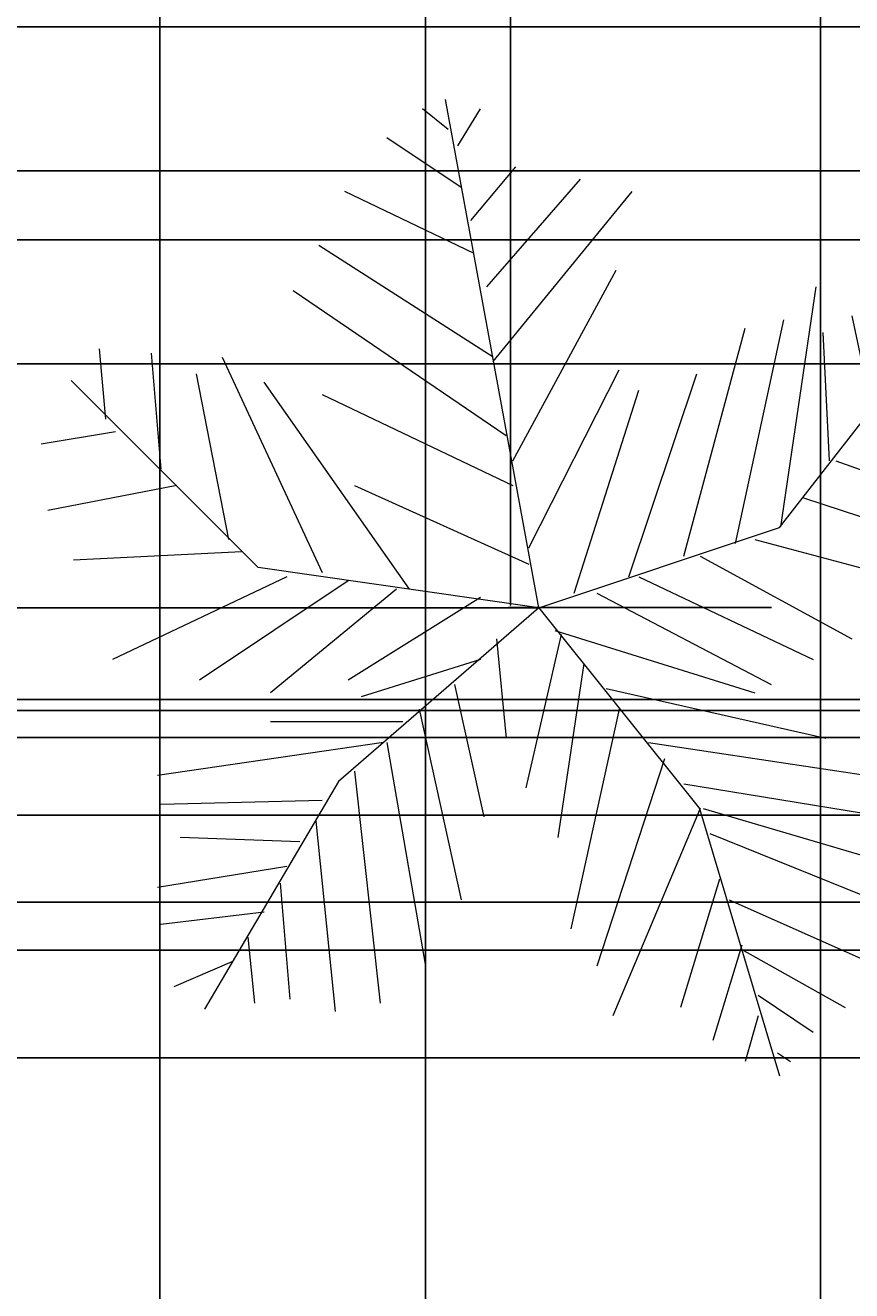
# Model space of a CAD drawing. Units: inches. Extents: x 818 to 1898, y 976 to 2364.
# Tile 10 of 96: x 1002 to 1071, y 1668 to 1773. Entities that reach past the tile are written whole.
import ezdxf

# ---------------------------------------------------------------- set-up
doc = ezdxf.new("R2010")
doc.units = ezdxf.units.IN
doc.header["$LTSCALE"] = 5
doc.header["$MEASUREMENT"] = 0
doc.layers.add('A-ANNO-DIMS', color=2, linetype='Continuous', lineweight=18)
doc.layers.add('L-PLNT', color=116, linetype='Continuous', lineweight=13, true_color=0x136734)
doc.styles.get("Standard").update_dxf_attribs({"font": 'arial.ttf'})
doc.dimstyles.get("Standard").update_dxf_attribs({"dimtxt": 0.18, "dimasz": 0.18, "dimexe": 0.18, "dimexo": 0.0625, "dimgap": 0.09, "dimtad": 0, "dimtih": 1, "dimtoh": 1, "dimdec": 4, "dimzin": 0, "dimdsep": 46, "dimtxsty": 'Standard', "dimcen": 0.09, "dimadec": 0, "dimazin": 0, "dimtfac": 1, "dimtdec": 4, "dimtofl": 0, "dimtmove": 0, "dimatfit": 3, "dimfxl": 1, "dimtolj": 1, "dimtzin": 0, "dimarcsym": 0})

# ---------------------------------------------------------------- blocks, each defined once
blk = doc.blocks.new('PALM-BORDER')
for p, q in [((41.53, 39.05), (33.72, 81.45)), ((33.95, 78.95), (31.8, 80.68)), ((34.76, 77.57), (36.65, 80.68)), ((35.03, 74.11), (28.83, 78.26)), ((35.84, 71.35), (39.61, 75.84)), ((37.18, 65.82), (45, 74.8)), ((36.11, 68.59), (25.33, 73.77)), ((37.72, 59.6), (49.31, 73.77)), ((37.72, 59.95), (23.17, 69.28)), ((39.34, 51.31), (47.96, 67.2)), ((38.8, 53.39), (21.02, 65.48)), ((61.61, 45.75), (77.23, 65.83)), ((61.71, 45.79), (64.67, 65.82)), ((74.37, 66.17), (75.18, 63.4)), ((70.33, 64.44), (72.75, 60.3)), ((67.63, 63.4), (69.25, 55.81)), ((53.62, 43.37), (58.74, 62.37)), ((57.93, 44.41), (61.97, 63.06)), ((65.21, 62.02), (65.75, 51.31)), ((74.1, 61.33), (79.49, 62.02)), ((5.39, 54.77), (4.85, 60.64)), ((9.16, 60.3), (9.97, 50.62)), ((15.09, 59.95), (23.44, 41.99)), ((12.93, 58.57), (15.63, 44.75)), ((40.69, 44.06), (48.23, 58.91)), ((49.04, 41.64), (54.7, 58.57)), ((71.68, 58.22), (77.87, 57.53)), ((18.1, 42.4), (2.48, 58.02)), ((30.72, 40.61), (18.59, 57.88)), ((44.46, 40.26), (49.85, 57.19)), ((23.44, 56.84), (39.34, 49.24)), ((6.2, 53.73), (0, 52.7)), ((68.44, 53.73), (77.33, 52.35)), ((66.29, 51.31), (77.87, 47.17)), ((11.32, 49.24), (0.54, 47.17)), ((26.14, 49.24), (40.69, 42.68)), ((63.59, 48.21), (77.33, 43.71)), ((41.53, 39.05), (61.61, 45.75)), ((59.55, 44.75), (76.26, 40.26)), ((16.71, 43.71), (2.69, 43.02)), ((54.97, 43.37), (67.63, 36.46)), ((41.53, 39.05), (18.1, 42.4)), ((20.48, 41.64), (5.93, 34.73)), ((25.6, 41.3), (13.2, 33.01)), ((49.85, 41.64), (64.4, 34.73)), ((29.64, 40.61), (19.13, 31.97)), ((46.35, 40.26), (60.9, 32.66)), ((36.65, 39.91), (25.6, 33.01)), ((41.53, 39.05), (24.79, 24.55)), ((41.53, 39.05), (54.92, 22.32)), ((42.84, 37.15), (59.55, 31.97)), ((37.99, 36.46), (38.8, 28.17)), ((43.38, 36.81), (40.42, 24.02)), ((36.65, 34.73), (26.68, 31.62)), ((45.27, 34.39), (43.11, 19.88)), ((34.49, 32.66), (36.92, 21.61)), ((47.15, 32.32), (65.48, 28.17)), ((31.53, 30.59), (35.03, 14.7)), ((48.23, 30.59), (44.19, 12.28)), ((30.18, 29.55), (19.13, 29.55)), ((28.56, 27.82), (9.7, 25.06)), ((28.83, 27.82), (32.07, 9.17)), ((50.66, 27.82), (68.98, 25.06)), ((52, 26.44), (46.35, 9.17)), ((26.14, 25.41), (28.29, 6.06)), ((24.79, 24.55), (13.63, 5.58)), ((53.62, 24.37), (68.44, 21.95)), ((23.44, 22.99), (9.97, 22.64)), ((54.97, 22.3), (47.69, 5.02)), ((54.92, 22.32), (61.61, 0)), ((55.24, 22.3), (71.68, 17.46)), ((22.9, 21.26), (24.52, 5.37)), ((55.78, 20.22), (70.33, 14.35)), ((21.56, 19.53), (11.59, 19.88)), ((20.48, 17.46), (9.7, 15.73)), ((19.94, 16.08), (20.75, 6.41)), ((56.59, 16.42), (53.35, 5.72)), ((57.39, 14.7), (70.6, 8.83)), ((18.59, 13.66), (9.97, 12.62)), ((17.24, 11.59), (17.78, 6.06)), ((58.47, 10.9), (56.05, 2.95)), ((15.9, 9.52), (11.05, 7.44)), ((58.47, 10.55), (67.09, 5.72)), ((59.82, 6.75), (64.4, 3.64)), ((59.82, 5.02), (58.74, 1.22)), ((61.44, 1.92), (62.51, 1.22))]:
    blk.add_line(p, q)
blk = doc.blocks.new('*D28')
at = {"layer": 'A-ANNO-DIMS', "color": 0, "lineweight": -2, "ltscale": 5, "transparency": 16777216}
for p, q in [((1064.25, 1870.18), (1042.3, 1870.18)), ((1042.48, 1870), (1042.48, 1797.61)), ((1042.48, 1724.84), (1042.48, 1797.24)), ((1064.25, 1724.66), (1042.3, 1724.66))]:
    blk.add_line(p, q, dxfattribs=at)
at = {"layer": 'A-ANNO-DIMS', "color": 0, "ltscale": 5, "transparency": 16777216}
for points in [[(1042.45, 1870), (1042.51, 1870), (1042.48, 1870.18)], [(1042.45, 1724.84), (1042.51, 1724.84), (1042.48, 1724.66)]]:
    blk.add_solid(points, dxfattribs=at)
at = {"layer": 'Defpoints', "color": 0, "ltscale": 5, "transparency": 16777216}
for p in [(1042.48, 1870.18), (1064.31, 1870.18), (1064.31, 1724.66)]:
    blk.add_point(p, dxfattribs=at)
at = {"layer": 'A-ANNO-DIMS', "color": 0, "ltscale": 5, "transparency": 16777216, "insert": (1042.48, 1797.42), "char_height": 0.18, "attachment_point": 5}
blk.add_mtext('\\A1;DECK PALM 146 TYP.', dxfattribs=at)
blk = doc.blocks.new('*D59')
at = {"layer": 'A-ANNO-DIMS', "color": 0, "lineweight": -2, "ltscale": 5, "transparency": 16777216}
for p, q in [((1251.64, 2300.39), (818.03, 2300.39)), ((818.21, 2300.21), (818.21, 1669.95)), ((818.21, 1039.32), (818.21, 1669.59)), ((896.05, 1039.14), (818.03, 1039.14))]:
    blk.add_line(p, q, dxfattribs=at)
at = {"layer": 'A-ANNO-DIMS', "color": 0, "ltscale": 5, "transparency": 16777216}
for points in [[(818.18, 2300.21), (818.24, 2300.21), (818.21, 2300.39)], [(818.18, 1039.32), (818.24, 1039.32), (818.21, 1039.14)]]:
    blk.add_solid(points, dxfattribs=at)
at = {"layer": 'Defpoints', "color": 0, "ltscale": 5, "transparency": 16777216}
for p in [(818.21, 2300.39), (1251.71, 2300.39), (896.11, 1039.14)]:
    blk.add_point(p, dxfattribs=at)
at = {"layer": 'A-ANNO-DIMS', "color": 0, "ltscale": 5, "transparency": 16777216, "insert": (818.21, 1669.77), "char_height": 0.18, "attachment_point": 5}
blk.add_mtext('\\A1;1261.2', dxfattribs=at)
blk = doc.blocks.new('*D79')
at = {"layer": 'A-ANNO-DIMS', "color": 0, "lineweight": -2, "ltscale": 5, "transparency": 16777216}
for p, q in [((992.73, 1203.03), (992.73, 2363.87)), ((992.91, 2363.69), (1032.01, 2363.69)), ((1071.55, 2363.69), (1032.44, 2363.69)), ((1071.73, 1203.03), (1071.73, 2363.87))]:
    blk.add_line(p, q, dxfattribs=at)
at = {"layer": 'A-ANNO-DIMS', "color": 0, "ltscale": 5, "transparency": 16777216}
for points in [[(992.91, 2363.72), (992.91, 2363.66), (992.73, 2363.69)], [(1071.55, 2363.72), (1071.55, 2363.66), (1071.73, 2363.69)]]:
    blk.add_solid(points, dxfattribs=at)
at = {"layer": 'Defpoints', "color": 0, "ltscale": 5, "transparency": 16777216}
for p in [(1071.73, 2363.69), (992.73, 1202.96), (1071.73, 1202.96)]:
    blk.add_point(p, dxfattribs=at)
at = {"layer": 'A-ANNO-DIMS', "color": 0, "ltscale": 5, "transparency": 16777216, "insert": (1032.23, 2363.69), "char_height": 0.18, "attachment_point": 5}
blk.add_mtext('\\A1;79', dxfattribs=at)
blk = doc.blocks.new('*D84')
at = {"layer": 'A-ANNO-DIMS', "color": 0, "lineweight": -2, "ltscale": 5, "transparency": 16777216}
for p, q in [((1197.66, 1700.08), (818.03, 1700.08)), ((818.21, 1699.9), (818.21, 1600.76)), ((818.21, 1501.26), (818.21, 1600.4)), ((1197.66, 1501.08), (818.03, 1501.08))]:
    blk.add_line(p, q, dxfattribs=at)
at = {"layer": 'A-ANNO-DIMS', "color": 0, "ltscale": 5, "transparency": 16777216}
for points in [[(818.18, 1699.9), (818.24, 1699.9), (818.21, 1700.08)], [(818.18, 1501.26), (818.24, 1501.26), (818.21, 1501.08)]]:
    blk.add_solid(points, dxfattribs=at)
at = {"layer": 'Defpoints', "color": 0, "ltscale": 5, "transparency": 16777216}
for p in [(818.21, 1700.08), (1197.73, 1700.08), (1197.73, 1501.08)]:
    blk.add_point(p, dxfattribs=at)
at = {"layer": 'A-ANNO-DIMS', "color": 0, "ltscale": 5, "transparency": 16777216, "insert": (818.21, 1600.58), "char_height": 0.18, "attachment_point": 5}
blk.add_mtext('\\A1;199', dxfattribs=at)
blk = doc.blocks.new('*D91')
at = {"layer": 'A-ANNO-DIMS', "color": 0, "lineweight": -2, "ltscale": 5, "transparency": 16777216}
for p, q in [((959.17, 1071.12), (959.17, 2363.87)), ((959.35, 2363.69), (985.8, 2363.69)), ((1013.04, 2363.69), (986.59, 2363.69)), ((1013.22, 1071.12), (1013.22, 2363.87))]:
    blk.add_line(p, q, dxfattribs=at)
at = {"layer": 'A-ANNO-DIMS', "color": 0, "ltscale": 5, "transparency": 16777216}
for points in [[(959.35, 2363.72), (959.35, 2363.66), (959.17, 2363.69)], [(1013.04, 2363.72), (1013.04, 2363.66), (1013.22, 2363.69)]]:
    blk.add_solid(points, dxfattribs=at)
at = {"layer": 'Defpoints', "color": 0, "ltscale": 5, "transparency": 16777216}
for p in [(1013.22, 2363.69), (959.17, 1071.06), (1013.22, 1071.06)]:
    blk.add_point(p, dxfattribs=at)
at = {"layer": 'A-ANNO-DIMS', "color": 0, "ltscale": 5, "transparency": 16777216, "insert": (986.2, 2363.69), "char_height": 0.18, "attachment_point": 5}
blk.add_mtext('\\A1;54.04', dxfattribs=at)
blk = doc.blocks.new('*D92')
at = {"layer": 'A-ANNO-DIMS', "color": 0, "lineweight": -2, "ltscale": 5, "transparency": 16777216}
for p, q in [((1013.22, 1071.12), (1013.22, 2363.87)), ((1013.4, 2363.69), (1040.38, 2363.69)), ((1068.16, 2363.69), (1041.17, 2363.69)), ((1068.34, 1071.12), (1068.34, 2363.87))]:
    blk.add_line(p, q, dxfattribs=at)
at = {"layer": 'A-ANNO-DIMS', "color": 0, "ltscale": 5, "transparency": 16777216}
for points in [[(1013.4, 2363.72), (1013.4, 2363.66), (1013.22, 2363.69)], [(1068.16, 2363.72), (1068.16, 2363.66), (1068.34, 2363.69)]]:
    blk.add_solid(points, dxfattribs=at)
at = {"layer": 'Defpoints', "color": 0, "ltscale": 5, "transparency": 16777216}
for p in [(1068.34, 2363.69), (1013.22, 1071.06), (1068.34, 1071.06)]:
    blk.add_point(p, dxfattribs=at)
at = {"layer": 'A-ANNO-DIMS', "color": 0, "ltscale": 5, "transparency": 16777216, "insert": (1040.78, 2363.69), "char_height": 0.18, "attachment_point": 5}
blk.add_mtext('\\A1;55.12', dxfattribs=at)
blk = doc.blocks.new('*D93')
at = {"layer": 'A-ANNO-DIMS', "color": 0, "lineweight": -2, "ltscale": 5, "transparency": 16777216}
for p, q in [((1068.34, 1071.12), (1068.34, 2363.87)), ((1068.52, 2363.69), (1094.16, 2363.69)), ((1120.58, 2363.69), (1094.94, 2363.69)), ((1120.76, 1071.12), (1120.76, 2363.87))]:
    blk.add_line(p, q, dxfattribs=at)
at = {"layer": 'A-ANNO-DIMS', "color": 0, "ltscale": 5, "transparency": 16777216}
for points in [[(1068.52, 2363.72), (1068.52, 2363.66), (1068.34, 2363.69)], [(1120.58, 2363.72), (1120.58, 2363.66), (1120.76, 2363.69)]]:
    blk.add_solid(points, dxfattribs=at)
at = {"layer": 'Defpoints', "color": 0, "ltscale": 5, "transparency": 16777216}
for p in [(1120.76, 2363.69), (1068.34, 1071.06), (1120.76, 1071.06)]:
    blk.add_point(p, dxfattribs=at)
at = {"layer": 'A-ANNO-DIMS', "color": 0, "ltscale": 5, "transparency": 16777216, "insert": (1094.55, 2363.69), "char_height": 0.18, "attachment_point": 5}
blk.add_mtext('\\A1;52.42', dxfattribs=at)
blk = doc.blocks.new('*D119')
at = {"layer": 'A-ANNO-DIMS', "color": 0, "lineweight": -2, "ltscale": 5, "transparency": 16777216}
for p, q in [((1766.29, 1716.99), (818.03, 1716.99)), ((818.21, 1716.81), (818.21, 1672.43)), ((818.21, 1627.69), (818.21, 1672.06)), ((1766.29, 1627.51), (818.03, 1627.51))]:
    blk.add_line(p, q, dxfattribs=at)
at = {"layer": 'A-ANNO-DIMS', "color": 0, "ltscale": 5, "transparency": 16777216}
for points in [[(818.18, 1716.81), (818.24, 1716.81), (818.21, 1716.99)], [(818.18, 1627.69), (818.24, 1627.69), (818.21, 1627.51)]]:
    blk.add_solid(points, dxfattribs=at)
at = {"layer": 'Defpoints', "color": 0, "ltscale": 5, "transparency": 16777216}
for p in [(818.21, 1716.99), (1766.35, 1716.99), (1766.35, 1627.51)]:
    blk.add_point(p, dxfattribs=at)
at = {"layer": 'A-ANNO-DIMS', "color": 0, "ltscale": 5, "transparency": 16777216, "insert": (818.21, 1672.25), "char_height": 0.18, "attachment_point": 5}
blk.add_mtext('\\A1;89.48', dxfattribs=at)
blk = doc.blocks.new('*D120')
at = {"layer": 'A-ANNO-DIMS', "color": 0, "lineweight": -2, "ltscale": 5, "transparency": 16777216}
for p, q in [((1766.29, 1797.72), (818.03, 1797.72)), ((818.21, 1797.54), (818.21, 1757.53)), ((818.21, 1717.17), (818.21, 1757.17)), ((1766.29, 1716.99), (818.03, 1716.99))]:
    blk.add_line(p, q, dxfattribs=at)
at = {"layer": 'A-ANNO-DIMS', "color": 0, "ltscale": 5, "transparency": 16777216}
for points in [[(818.18, 1797.54), (818.24, 1797.54), (818.21, 1797.72)], [(818.18, 1717.17), (818.24, 1717.17), (818.21, 1716.99)]]:
    blk.add_solid(points, dxfattribs=at)
at = {"layer": 'Defpoints', "color": 0, "ltscale": 5, "transparency": 16777216}
for p in [(818.21, 1797.72), (1766.35, 1797.72), (1766.35, 1716.99)]:
    blk.add_point(p, dxfattribs=at)
at = {"layer": 'A-ANNO-DIMS', "color": 0, "ltscale": 5, "transparency": 16777216, "insert": (818.21, 1757.35), "char_height": 0.18, "attachment_point": 5}
blk.add_mtext('\\A1;80.73', dxfattribs=at)
blk = doc.blocks.new('*D126')
at = {"layer": 'A-ANNO-DIMS', "color": 0, "lineweight": -2, "ltscale": 5, "transparency": 16777216}
for p, q in [((1035.38, 1252.09), (1035.38, 2363.87)), ((1035.56, 2363.69), (1075.41, 2363.69)), ((1116.01, 2363.69), (1076.16, 2363.69)), ((1116.19, 1236.03), (1116.19, 2363.87))]:
    blk.add_line(p, q, dxfattribs=at)
at = {"layer": 'A-ANNO-DIMS', "color": 0, "ltscale": 5, "transparency": 16777216}
for points in [[(1035.56, 2363.72), (1035.56, 2363.66), (1035.38, 2363.69)], [(1116.01, 2363.72), (1116.01, 2363.66), (1116.19, 2363.69)]]:
    blk.add_solid(points, dxfattribs=at)
at = {"layer": 'Defpoints', "color": 0, "ltscale": 5, "transparency": 16777216}
for p in [(1035.38, 2363.69), (1035.38, 1252.02), (1116.19, 1235.96)]:
    blk.add_point(p, dxfattribs=at)
at = {"layer": 'A-ANNO-DIMS', "color": 0, "ltscale": 5, "transparency": 16777216, "insert": (1075.78, 2363.69), "char_height": 0.18, "attachment_point": 5}
blk.add_mtext('\\A1;80.81', dxfattribs=at)
blk = doc.blocks.new('*D130')
at = {"layer": 'A-ANNO-DIMS', "color": 0, "lineweight": -2, "ltscale": 5, "transparency": 16777216}
for p, q in [((1044.78, 1724.63), (818.03, 1724.63)), ((818.21, 1724.45), (818.21, 1666.75)), ((818.21, 1608.69), (818.21, 1666.39)), ((1044.78, 1608.51), (818.03, 1608.51))]:
    blk.add_line(p, q, dxfattribs=at)
at = {"layer": 'A-ANNO-DIMS', "color": 0, "ltscale": 5, "transparency": 16777216}
for points in [[(818.18, 1724.45), (818.24, 1724.45), (818.21, 1724.63)], [(818.18, 1608.69), (818.24, 1608.69), (818.21, 1608.51)]]:
    blk.add_solid(points, dxfattribs=at)
at = {"layer": 'Defpoints', "color": 0, "ltscale": 5, "transparency": 16777216}
for p in [(818.21, 1724.63), (1044.85, 1724.63), (1044.85, 1608.51)]:
    blk.add_point(p, dxfattribs=at)
at = {"layer": 'A-ANNO-DIMS', "color": 0, "ltscale": 5, "transparency": 16777216, "insert": (818.21, 1666.57), "char_height": 0.18, "attachment_point": 5}
blk.add_mtext('\\A1;116.12', dxfattribs=at)
blk = doc.blocks.new('*D131')
at = {"layer": 'A-ANNO-DIMS', "color": 0, "lineweight": -2, "ltscale": 5, "transparency": 16777216}
for p, q in [((1043.71, 1886.9), (818.03, 1886.9)), ((818.21, 1886.72), (818.21, 1805.95)), ((818.21, 1724.81), (818.21, 1805.58)), ((1044.78, 1724.63), (818.03, 1724.63))]:
    blk.add_line(p, q, dxfattribs=at)
at = {"layer": 'A-ANNO-DIMS', "color": 0, "ltscale": 5, "transparency": 16777216}
for points in [[(818.18, 1886.72), (818.24, 1886.72), (818.21, 1886.9)], [(818.18, 1724.81), (818.24, 1724.81), (818.21, 1724.63)]]:
    blk.add_solid(points, dxfattribs=at)
at = {"layer": 'Defpoints', "color": 0, "ltscale": 5, "transparency": 16777216}
for p in [(818.21, 1886.9), (1043.77, 1886.9), (1044.85, 1724.63)]:
    blk.add_point(p, dxfattribs=at)
at = {"layer": 'A-ANNO-DIMS', "color": 0, "ltscale": 5, "transparency": 16777216, "insert": (818.21, 1805.77), "char_height": 0.18, "attachment_point": 5}
blk.add_mtext('\\A1;162.27', dxfattribs=at)
blk = doc.blocks.new('*D176')
at = {"layer": 'A-ANNO-DIMS', "color": 0, "lineweight": -2, "ltscale": 5, "transparency": 16777216}
for p, q in [((1559.66, 1687.08), (818.03, 1687.08)), ((818.21, 1686.9), (818.21, 1667.51)), ((818.21, 1647.76), (818.21, 1667.15)), ((1559.66, 1647.58), (818.03, 1647.58))]:
    blk.add_line(p, q, dxfattribs=at)
at = {"layer": 'A-ANNO-DIMS', "color": 0, "ltscale": 5, "transparency": 16777216}
for points in [[(818.18, 1686.9), (818.24, 1686.9), (818.21, 1687.08)], [(818.18, 1647.76), (818.24, 1647.76), (818.21, 1647.58)]]:
    blk.add_solid(points, dxfattribs=at)
at = {"layer": 'Defpoints', "color": 0, "ltscale": 5, "transparency": 16777216}
for p in [(1559.73, 1687.08), (818.21, 1647.58), (1559.73, 1647.58)]:
    blk.add_point(p, dxfattribs=at)
at = {"layer": 'A-ANNO-DIMS', "color": 0, "ltscale": 5, "transparency": 16777216, "insert": (818.21, 1667.33), "char_height": 0.18, "attachment_point": 5}
blk.add_mtext('\\A1;39.5', dxfattribs=at)
blk = doc.blocks.new('*D215')
at = {"layer": 'A-ANNO-DIMS', "color": 0, "lineweight": -2, "ltscale": 5, "transparency": 16777216}
for p, q in [((1590.66, 1876.08), (818.03, 1876.08)), ((818.21, 1875.9), (818.21, 1781.76)), ((818.21, 1687.26), (818.21, 1781.4)), ((1511.66, 1687.08), (818.03, 1687.08))]:
    blk.add_line(p, q, dxfattribs=at)
at = {"layer": 'A-ANNO-DIMS', "color": 0, "ltscale": 5, "transparency": 16777216}
for points in [[(818.18, 1875.9), (818.24, 1875.9), (818.21, 1876.08)], [(818.18, 1687.26), (818.24, 1687.26), (818.21, 1687.08)]]:
    blk.add_solid(points, dxfattribs=at)
at = {"layer": 'Defpoints', "color": 0, "ltscale": 5, "transparency": 16777216}
for p in [(818.21, 1876.08), (1590.73, 1876.08), (1511.73, 1687.08)]:
    blk.add_point(p, dxfattribs=at)
at = {"layer": 'A-ANNO-DIMS', "color": 0, "ltscale": 5, "transparency": 16777216, "insert": (818.21, 1781.58), "char_height": 0.18, "attachment_point": 5}
blk.add_mtext('\\A1;189', dxfattribs=at)
blk = doc.blocks.new('*D220')
at = {"layer": 'A-ANNO-DIMS', "color": 0, "lineweight": -2, "ltscale": 5, "transparency": 16777216}
for p, q in [((1520.66, 1773.08), (818.03, 1773.08)), ((818.21, 1772.9), (818.21, 1767.26)), ((818.21, 1761.26), (818.21, 1766.9)), ((1520.66, 1761.08), (818.03, 1761.08))]:
    blk.add_line(p, q, dxfattribs=at)
at = {"layer": 'A-ANNO-DIMS', "color": 0, "ltscale": 5, "transparency": 16777216}
for points in [[(818.18, 1772.9), (818.24, 1772.9), (818.21, 1773.08)], [(818.18, 1761.26), (818.24, 1761.26), (818.21, 1761.08)]]:
    blk.add_solid(points, dxfattribs=at)
at = {"layer": 'Defpoints', "color": 0, "ltscale": 5, "transparency": 16777216}
for p in [(818.21, 1773.08), (1520.73, 1773.08), (1520.73, 1761.08)]:
    blk.add_point(p, dxfattribs=at)
at = {"layer": 'A-ANNO-DIMS', "color": 0, "ltscale": 5, "transparency": 16777216, "insert": (818.21, 1767.08), "char_height": 0.18, "attachment_point": 5}
blk.add_mtext('\\A1;12', dxfattribs=at)
blk = doc.blocks.new('*D222')
at = {"layer": 'A-ANNO-DIMS', "color": 0, "lineweight": -2, "ltscale": 5, "transparency": 16777216}
for p, q in [((1511.66, 1744.97), (818.03, 1744.97)), ((818.21, 1744.79), (818.21, 1730.69)), ((818.21, 1716.23), (818.21, 1730.33)), ((1511.66, 1716.05), (818.03, 1716.05))]:
    blk.add_line(p, q, dxfattribs=at)
at = {"layer": 'A-ANNO-DIMS', "color": 0, "ltscale": 5, "transparency": 16777216}
for points in [[(818.18, 1744.79), (818.24, 1744.79), (818.21, 1744.97)], [(818.18, 1716.23), (818.24, 1716.23), (818.21, 1716.05)]]:
    blk.add_solid(points, dxfattribs=at)
at = {"layer": 'Defpoints', "color": 0, "ltscale": 5, "transparency": 16777216}
for p in [(818.21, 1744.97), (1511.73, 1744.97), (1511.73, 1716.05)]:
    blk.add_point(p, dxfattribs=at)
at = {"layer": 'A-ANNO-DIMS', "color": 0, "ltscale": 5, "transparency": 16777216, "insert": (818.21, 1730.51), "char_height": 0.18, "attachment_point": 5}
blk.add_mtext('\\A1;28.926', dxfattribs=at)
blk = doc.blocks.new('*D223')
at = {"layer": 'A-ANNO-DIMS', "color": 0, "lineweight": -2, "ltscale": 5, "transparency": 16777216}
for p, q in [((1511.66, 1716.05), (818.03, 1716.05)), ((818.21, 1715.87), (818.21, 1706.24)), ((818.21, 1696.26), (818.21, 1705.88)), ((1511.66, 1696.08), (818.03, 1696.08))]:
    blk.add_line(p, q, dxfattribs=at)
at = {"layer": 'A-ANNO-DIMS', "color": 0, "ltscale": 5, "transparency": 16777216}
for points in [[(818.18, 1715.87), (818.24, 1715.87), (818.21, 1716.05)], [(818.18, 1696.26), (818.24, 1696.26), (818.21, 1696.08)]]:
    blk.add_solid(points, dxfattribs=at)
at = {"layer": 'Defpoints', "color": 0, "ltscale": 5, "transparency": 16777216}
for p in [(818.21, 1716.05), (1511.73, 1716.05), (1511.73, 1696.08)]:
    blk.add_point(p, dxfattribs=at)
at = {"layer": 'A-ANNO-DIMS', "color": 0, "ltscale": 5, "transparency": 16777216, "insert": (818.21, 1706.06), "char_height": 0.18, "attachment_point": 5}
blk.add_mtext('\\A1;19.967', dxfattribs=at)
blk = doc.blocks.new('*D246')
at = {"layer": 'A-ANNO-DIMS', "color": 0, "lineweight": -2, "ltscale": 5, "transparency": 16777216}
for p, q in [((1258.66, 1755.33), (818.03, 1755.33)), ((818.21, 1755.15), (818.21, 1731.51)), ((818.21, 1707.51), (818.21, 1731.15)), ((1258.66, 1707.33), (818.03, 1707.33))]:
    blk.add_line(p, q, dxfattribs=at)
at = {"layer": 'A-ANNO-DIMS', "color": 0, "ltscale": 5, "transparency": 16777216}
for points in [[(818.18, 1755.15), (818.24, 1755.15), (818.21, 1755.33)], [(818.18, 1707.51), (818.24, 1707.51), (818.21, 1707.33)]]:
    blk.add_solid(points, dxfattribs=at)
at = {"layer": 'Defpoints', "color": 0, "ltscale": 5, "transparency": 16777216}
for p in [(818.21, 1755.33), (1258.73, 1755.33), (1258.73, 1707.33)]:
    blk.add_point(p, dxfattribs=at)
at = {"layer": 'A-ANNO-DIMS', "color": 0, "ltscale": 5, "transparency": 16777216, "insert": (818.21, 1731.33), "char_height": 0.18, "attachment_point": 5}
blk.add_mtext('\\A1;48', dxfattribs=at)
blk = doc.blocks.new('*D249')
at = {"layer": 'A-ANNO-DIMS', "color": 0, "lineweight": -2, "ltscale": 5, "transparency": 16777216}
for p, q in [((1258.66, 1814.97), (818.03, 1814.97)), ((818.21, 1814.79), (818.21, 1785.33)), ((818.21, 1755.51), (818.21, 1784.97)), ((1258.66, 1755.33), (818.03, 1755.33))]:
    blk.add_line(p, q, dxfattribs=at)
at = {"layer": 'A-ANNO-DIMS', "color": 0, "ltscale": 5, "transparency": 16777216}
for points in [[(818.18, 1814.79), (818.24, 1814.79), (818.21, 1814.97)], [(818.18, 1755.51), (818.24, 1755.51), (818.21, 1755.33)]]:
    blk.add_solid(points, dxfattribs=at)
at = {"layer": 'Defpoints', "color": 0, "ltscale": 5, "transparency": 16777216}
for p in [(818.21, 1814.97), (1258.73, 1814.97), (1258.73, 1755.33)]:
    blk.add_point(p, dxfattribs=at)
at = {"layer": 'A-ANNO-DIMS', "color": 0, "ltscale": 5, "transparency": 16777216, "insert": (818.21, 1785.15), "char_height": 0.18, "attachment_point": 5}
blk.add_mtext('\\A1;59.63', dxfattribs=at)
blk = doc.blocks.new('*D277')
at = {"layer": 'A-ANNO-DIMS', "color": 0, "lineweight": -2, "ltscale": 5, "transparency": 16777216}
for p, q in [((1251.87, 1687.08), (818.03, 1687.08)), ((818.21, 1686.9), (818.21, 1668.7)), ((818.21, 1650.13), (818.21, 1668.33)), ((1256.59, 1649.95), (818.03, 1649.95))]:
    blk.add_line(p, q, dxfattribs=at)
at = {"layer": 'A-ANNO-DIMS', "color": 0, "ltscale": 5, "transparency": 16777216}
for points in [[(818.18, 1686.9), (818.24, 1686.9), (818.21, 1687.08)], [(818.18, 1650.13), (818.24, 1650.13), (818.21, 1649.95)]]:
    blk.add_solid(points, dxfattribs=at)
at = {"layer": 'Defpoints', "color": 0, "ltscale": 5, "transparency": 16777216}
for p in [(818.21, 1687.08), (1251.93, 1687.08), (1256.65, 1649.95)]:
    blk.add_point(p, dxfattribs=at)
at = {"layer": 'A-ANNO-DIMS', "color": 0, "ltscale": 5, "transparency": 16777216, "insert": (818.21, 1668.52), "char_height": 0.18, "attachment_point": 5}
blk.add_mtext('\\A1;37.13', dxfattribs=at)
blk = doc.blocks.new('*D289')
at = {"layer": 'A-ANNO-DIMS', "color": 0, "lineweight": -2, "ltscale": 5, "transparency": 16777216}
for p, q in [((1279.06, 1713.82), (818.03, 1713.82)), ((818.21, 1713.64), (818.21, 1705.13)), ((818.21, 1696.26), (818.21, 1704.77)), ((1267.66, 1696.08), (818.03, 1696.08))]:
    blk.add_line(p, q, dxfattribs=at)
at = {"layer": 'A-ANNO-DIMS', "color": 0, "ltscale": 5, "transparency": 16777216}
for points in [[(818.18, 1713.64), (818.24, 1713.64), (818.21, 1713.82)], [(818.18, 1696.26), (818.24, 1696.26), (818.21, 1696.08)]]:
    blk.add_solid(points, dxfattribs=at)
at = {"layer": 'Defpoints', "color": 0, "ltscale": 5, "transparency": 16777216}
for p in [(1279.13, 1713.82), (818.21, 1696.08), (1267.73, 1696.08)]:
    blk.add_point(p, dxfattribs=at)
at = {"layer": 'A-ANNO-DIMS', "color": 0, "ltscale": 5, "transparency": 16777216, "insert": (818.21, 1704.95), "char_height": 0.18, "attachment_point": 5}
blk.add_mtext('\\A1;17.74', dxfattribs=at)

msp = doc.modelspace()

# ---------------------------------------------------------------- block references
at = {"layer": 'L-PLNT'}
msp.add_blockref('PALM-BORDER', (1003.3185, 1685.5789), dxfattribs=at)

# ---------------------------------------------------------------- dimensions: what is measured, and where the dimension line sits
at = {"layer": 'A-ANNO-DIMS', "ltscale": 5}
for base, p1, p2, override, picture, middle in [((1013.2176, 2363.6929), (959.1737, 1071.0552), (1013.2176, 1071.0552), {"dimdec": 2, "dimlfac": 1, "dimrnd": 0, "dimzin": 0, "dimdsep": 46, "dimlunit": 2}, '*D91', (986.1956, 2363.6929)), ((1071.7251, 2363.6929), (992.7251, 1202.9642), (1071.7251, 1202.9642), {"dimdec": 0, "dimlfac": 1, "dimrnd": 0, "dimzin": 0, "dimdsep": 46, "dimlunit": 2}, '*D79', (1032.2251, 2363.6929)), ((1068.3377, 2363.6929), (1013.2176, 1071.0552), (1068.3377, 1071.0552), {"dimdec": 2, "dimlfac": 1, "dimrnd": 0, "dimzin": 0, "dimdsep": 46, "dimlunit": 2}, '*D92', (1040.7776, 2363.6929)), ((1035.3768, 2363.6929), (1116.1882, 1235.9642), (1035.3768, 1252.0242), {"dimdec": 2, "dimlfac": 1, "dimrnd": 0, "dimzin": 0, "dimdsep": 46, "dimlunit": 2}, '*D126', (1075.7825, 2363.6929)), ((1120.7618, 2363.6929), (1068.3377, 1071.0552), (1120.7618, 1071.0552), {"dimdec": 2, "dimlfac": 1, "dimrnd": 0, "dimzin": 0, "dimdsep": 46, "dimlunit": 2}, '*D93', (1094.5497, 2363.6929))]:
    dim = msp.add_linear_dim(base=base, p1=p1, p2=p2, dimstyle='Standard', override=override, dxfattribs=at)
    dim.commit()
    dim.dimension.update_dxf_attribs({"geometry": picture, "text_midpoint": middle})
for base, p1, p2, override, picture, middle in [((818.2059, 2300.3929), (896.1138, 1039.1433), (1251.7057, 2300.3929), {"dimdec": 1, "dimlfac": 1, "dimrnd": 0, "dimzin": 0, "dimdsep": 46, "dimlunit": 2}, '*D59', (818.2059, 1669.7681)), ((818.2059, 1886.9018), (1044.8463, 1724.63), (1043.7685, 1886.9018), {"dimdec": 2, "dimlfac": 1, "dimrnd": 0, "dimzin": 0, "dimdsep": 46, "dimlunit": 2}, '*D131', (818.2059, 1805.7659)), ((818.2059, 1876.0782), (1511.7251, 1687.0782), (1590.7251, 1876.0782), {"dimdec": 0, "dimlfac": 1, "dimrnd": 0, "dimzin": 0, "dimdsep": 46, "dimlunit": 2}, '*D215', (818.2059, 1781.5782)), ((818.2059, 1814.9652), (1258.7251, 1755.3321), (1258.7251, 1814.9652), {"dimdec": 2, "dimlfac": 1, "dimrnd": 0, "dimzin": 0, "dimdsep": 46, "dimlunit": 2}, '*D249', (818.2059, 1785.1486)), ((818.2059, 1797.7165), (1766.3524, 1716.9866), (1766.3524, 1797.7165), {"dimdec": 2, "dimlfac": 1, "dimrnd": 0, "dimzin": 0, "dimdsep": 46, "dimlunit": 2}, '*D120', (818.2059, 1757.3516)), ((818.2059, 1773.0782), (1520.7251, 1761.0782), (1520.7251, 1773.0782), {"dimdec": 0, "dimlfac": 1, "dimrnd": 0, "dimzin": 0, "dimdsep": 46, "dimlunit": 2}, '*D220', (818.2059, 1767.0782)), ((818.2059, 1755.3321), (1258.7251, 1707.3321), (1258.7251, 1755.3321), {"dimdec": 0, "dimlfac": 1, "dimrnd": 0, "dimzin": 0, "dimdsep": 46, "dimlunit": 2}, '*D246', (818.2059, 1731.3321)), ((818.2059, 1744.9714), (1511.7251, 1716.0454), (1511.7251, 1744.9714), {"dimdec": 3, "dimlfac": 1, "dimrnd": 0, "dimzin": 0, "dimdsep": 46, "dimlunit": 2}, '*D222', (818.2059, 1730.5084)), ((818.2059, 1724.63), (1044.8463, 1608.5116), (1044.8463, 1724.63), {"dimdec": 2, "dimlfac": 1, "dimrnd": 0, "dimzin": 0, "dimdsep": 46, "dimlunit": 2}, '*D130', (818.2059, 1666.5708)), ((818.2059, 1716.9866), (1766.3524, 1627.5052), (1766.3524, 1716.9866), {"dimdec": 2, "dimlfac": 1, "dimrnd": 0, "dimzin": 0, "dimdsep": 46, "dimlunit": 2}, '*D119', (818.2059, 1672.2459)), ((818.2059, 1716.0454), (1511.7251, 1696.0782), (1511.7251, 1716.0454), {"dimdec": 3, "dimlfac": 1, "dimrnd": 0, "dimzin": 0, "dimdsep": 46, "dimlunit": 2}, '*D223', (818.2059, 1706.0618)), ((818.2059, 1696.0782), (1279.1253, 1713.8174), (1267.7251, 1696.0782), {"dimdec": 2, "dimlfac": 1, "dimrnd": 0, "dimzin": 0, "dimdsep": 46, "dimlunit": 2}, '*D289', (818.2059, 1704.9478)), ((818.2059, 1700.0782), (1197.7251, 1501.0782), (1197.7251, 1700.0782), {"dimdec": 0, "dimlfac": 1, "dimrnd": 0, "dimzin": 0, "dimdsep": 46, "dimlunit": 2}, '*D84', (818.2059, 1600.5782)), ((818.2059, 1687.0782), (1256.6519, 1649.9518), (1251.9333, 1687.0782), {"dimdec": 2, "dimlfac": 1, "dimrnd": 0, "dimzin": 0, "dimdsep": 46, "dimlunit": 2}, '*D277', (818.2059, 1668.515)), ((818.2059, 1647.5782), (1559.7251, 1687.0782), (1559.7251, 1647.5782), {"dimdec": 1, "dimlfac": 1, "dimrnd": 0, "dimzin": 0, "dimdsep": 46, "dimlunit": 2}, '*D176', (818.2059, 1667.3282))]:
    dim = msp.add_linear_dim(base=base, p1=p1, p2=p2, angle=90, dimstyle='Standard', override=override, dxfattribs=at)
    dim.commit()
    dim.dimension.update_dxf_attribs({"geometry": picture, "text_midpoint": middle})
dim = msp.add_linear_dim(base=(1042.4825, 1870.1814), p1=(1064.3101, 1724.6639), p2=(1064.3101, 1870.1814), angle=90, text='DECK PALM <> TYP.', dimstyle='Standard', override={"dimdec": 0, "dimlfac": 1, "dimrnd": 0, "dimzin": 0, "dimdsep": 46, "dimlunit": 2}, dxfattribs=at)
dim.commit()
dim.dimension.update_dxf_attribs({"geometry": '*D28', "text_midpoint": (1042.4825, 1797.4226)})

doc.saveas('drawing.dxf')
